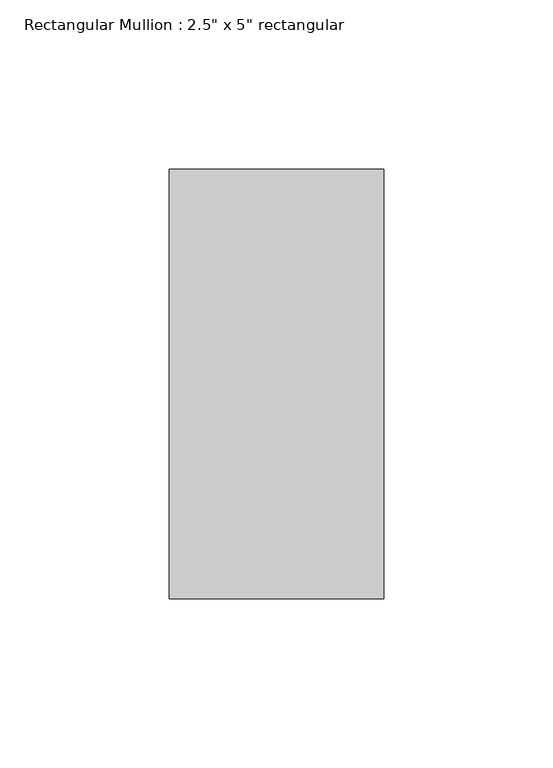
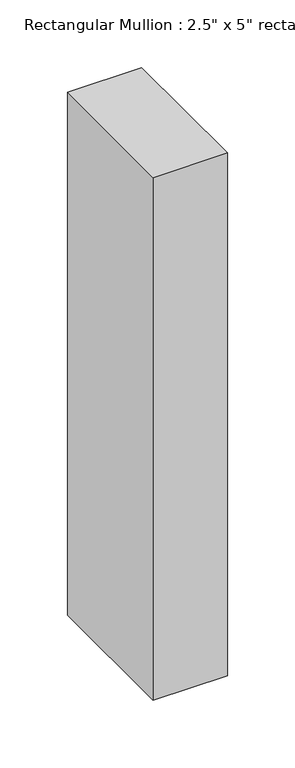
"""IFC4 building model written with IfcOpenShell, lengths in millimetres: member geometry."""

from ifc_helpers import new_model, si_unit, frame, origin, place, context, project, spatial, polyline, outline, extrude, source, transform, mapped, element, save


def member_0af91ce1(model_context):
    return source(origin(), model_context, "Body", "SweptSolid", [
        extrude(outline(polyline([(0.0, 63.5), (0.0, -63.5), (-63.5, -63.5), (-63.5, 63.5), (0.0, 63.5)])), frame((0.0, 0.0, -472.0166667), z_axis=(0.0, 0.0, 1.0), x_axis=(1.0, 0.0, 0.0)), (0.0, 0.0, 1.0), 472.0166667),
    ])


if __name__ == "__main__":
    model = new_model("IFC4")
    model_context = context("Model", 3, world=origin())
    ifc_project = project(units=[si_unit("LENGTHUNIT", "METRE", prefix="MILLI")], contexts=[model_context])
    site = spatial("IfcSite", under=ifc_project)
    building = spatial("IfcBuilding", under=site)
    placement = place(None, origin())
    member_shape = member_0af91ce1(model_context)
    element("IfcMember", 1, ObjectType="Rectangular Mullion : 2.5\" x 5\" rectangular", at=placement, inside=building, context=model_context, shape_type="MappedRepresentation", body=[
        mapped(member_shape, transform((0.0, 0.0, 0.0), x_axis=(1.0, 0.0, 0.0), y_axis=(0.0, 1.0, 0.0), z_axis=(0.0, 0.0, 1.0))),
    ])
    save(model, "model.ifc")

# Revit data of these elements
# Type "Rectangular Mullion : 2.5\" x 5\" rectangular"
#   built-in parameter 1007304 = 0.416667 (stored number, unit not read)
#   built-in parameter 1007301 = 0.104167 (stored number, unit not read)
#   built-in parameter 1007300 = 0.104167 (stored number, unit not read)
# Element 1 (IfcMember, "Rectangular Mullion : 2.5\" x 5\" rectangular")
#   Materials on its faces: "Aluminum"
# Materials
#   "Aluminum": class "Metal", colour RGB 247 247 247, transparency 0, Description = "Aluminum 6061", Cost = 0
